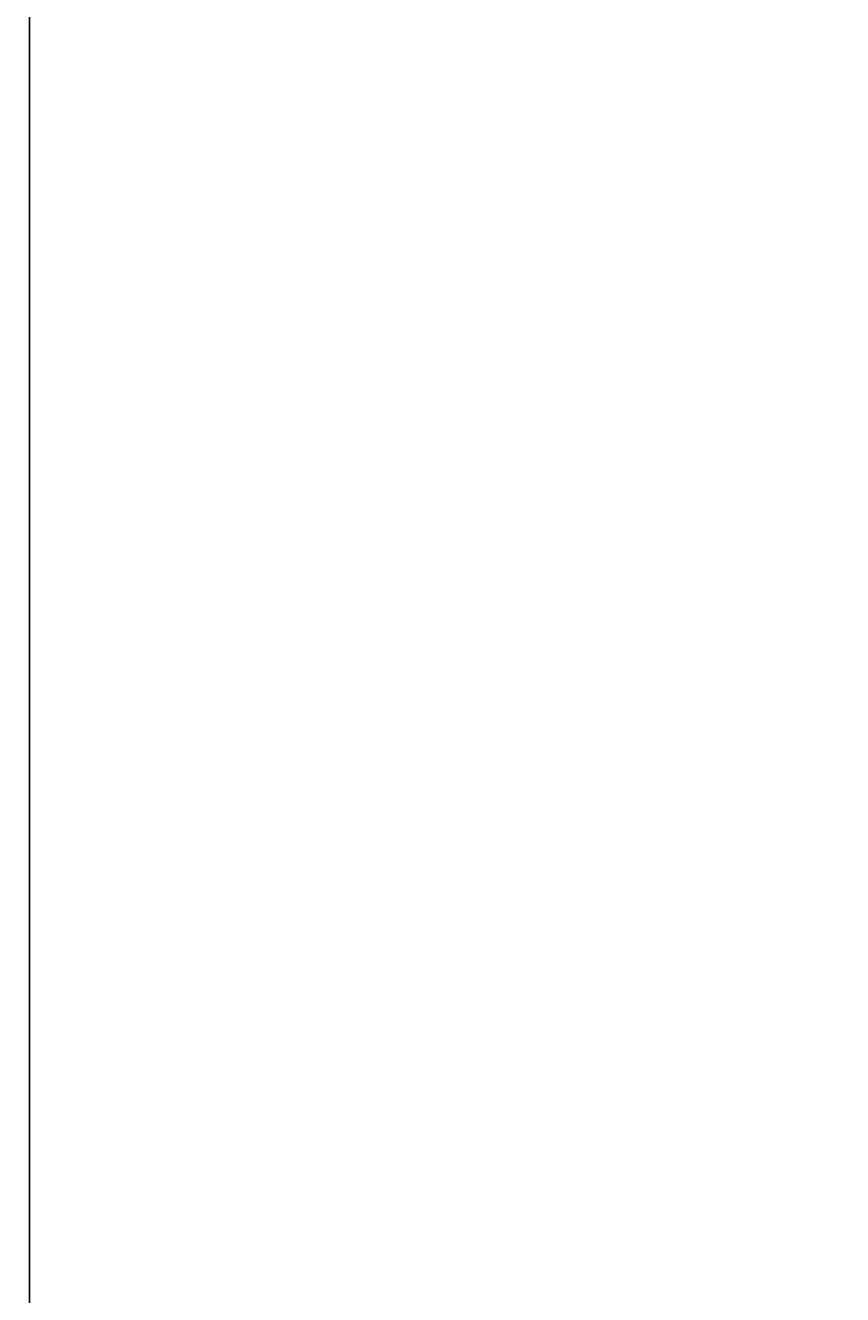
# Model space of a CAD drawing. Units: millimetres. Extents: x 27017497 to 27018854, y 7058029 to 7059154.
# Tile 9 of 91: x 27017497 to 27017560, y 7058200 to 7058297. Entities that reach past the tile are written whole.
import ezdxf

# ---------------------------------------------------------------- set-up
doc = ezdxf.new("R2010")
doc.units = ezdxf.units.MM
doc.layers.add('A-ANNO-DIMS', color=2, linetype='Continuous', lineweight=18)
doc.styles.get("Standard").update_dxf_attribs({"font": 'arial.ttf'})
doc.dimstyles.get("Standard").update_dxf_attribs({"dimtxt": 0.18, "dimasz": 0.18, "dimexe": 0.18, "dimexo": 0.0625, "dimgap": 0.09, "dimtad": 0, "dimtih": 1, "dimtoh": 1, "dimdec": 4, "dimzin": 0, "dimdsep": 46, "dimtxsty": 'Standard', "dimcen": 0.09, "dimadec": 0, "dimazin": 0, "dimtfac": 1, "dimtdec": 4, "dimtofl": 0, "dimtmove": 0, "dimatfit": 3, "dimfxl": 1, "dimtolj": 1, "dimtzin": 0, "dimarcsym": 0})

# ---------------------------------------------------------------- blocks, each defined once
blk = doc.blocks.new('*D48')
at = {"layer": 'A-ANNO-DIMS', "color": 0, "lineweight": -2, "transparency": 16777216}
for p, q in [((27018463.498, 7058622.912), (27017497.536, 7058622.912)), ((27017497.716, 7058622.732), (27017497.716, 7058357.753)), ((27017497.716, 7058092.41), (27017497.716, 7058357.389)), ((27018555.129, 7058092.23), (27017497.536, 7058092.23))]:
    blk.add_line(p, q, dxfattribs=at)
at = {"layer": 'A-ANNO-DIMS', "color": 0, "transparency": 16777216}
for points in [[(27017497.686, 7058622.732), (27017497.746, 7058622.732), (27017497.716, 7058622.912)], [(27017497.686, 7058092.41), (27017497.746, 7058092.41), (27017497.716, 7058092.23)]]:
    blk.add_solid(points, dxfattribs=at)
at = {"layer": 'Defpoints', "color": 0, "transparency": 16777216}
for p in [(27018463.561, 7058622.912), (27017497.716, 7058092.23), (27018555.192, 7058092.23)]:
    blk.add_point(p, dxfattribs=at)
at = {"layer": 'A-ANNO-DIMS', "color": 0, "transparency": 16777216, "insert": (27017497.716, 7058357.571), "char_height": 0.18, "attachment_point": 5}
blk.add_mtext('\\A1;530.7', dxfattribs=at)

msp = doc.modelspace()

# ---------------------------------------------------------------- dimensions: what is measured, and where the dimension line sits
at = {"layer": 'A-ANNO-DIMS'}
dim = msp.add_linear_dim(base=(27017497.716, 7058092.23), p1=(27018463.561, 7058622.912), p2=(27018555.192, 7058092.23), angle=90, dimstyle='Standard', override={"dimdec": 1, "dimlfac": 1, "dimrnd": 0, "dimzin": 0, "dimdsep": 46, "dimlunit": 2}, dxfattribs=at)
dim.commit()
dim.dimension.update_dxf_attribs({"geometry": '*D48', "text_midpoint": (27017497.716, 7058357.571)})

doc.saveas('drawing.dxf')
